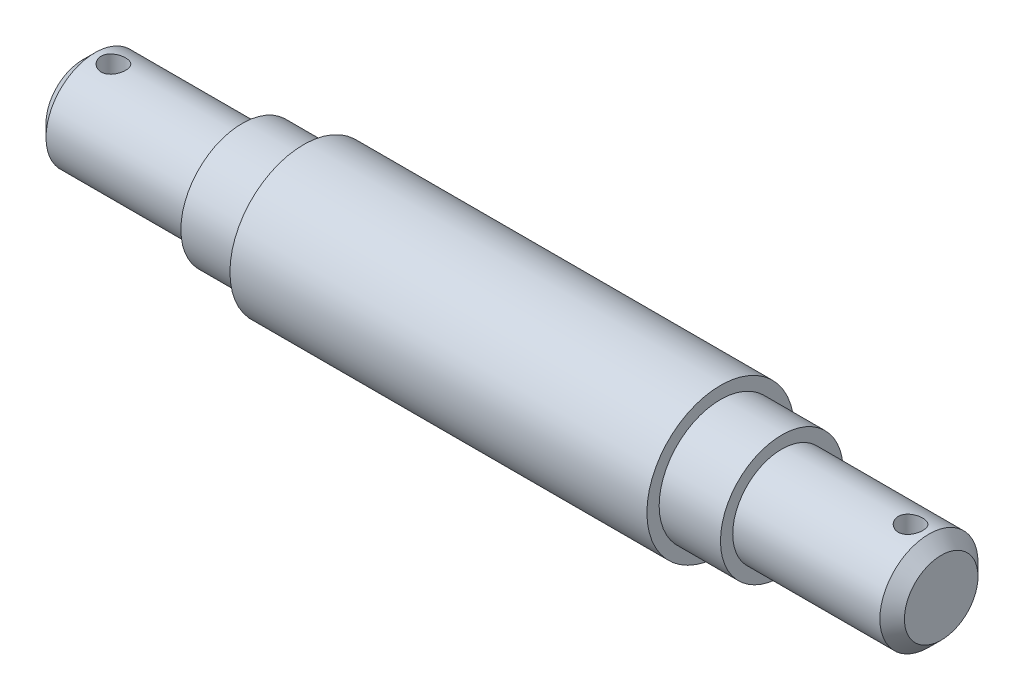
SolidWorks part; units mm, degrees
material "Plain Carbon Steel"
ref_plane "Front Plane" through (0, 0, 0) normal (0, 0, 1) x (1, 0, 0)
ref_plane "Top Plane" through (0, 0, 0) normal (0, 1, 0) x (1, 0, 0)
ref_plane "Right Plane" through (0, 0, 0) normal (1, 0, 0) x (0, 0, -1)
sketch "Shaft Profile Sketch" plane through (0, 0, 0) normal (0, 0, 1) x (1, 0, 0)
  line L0 (0, 0) -> (70, 0)
  line L1 (70, 0) -> (70, -4)
  line L2 (70, -4) -> (57, -4)
  line L3 (57, -4) -> (57, -5)
  line L4 (57, -5) -> (52, -5)
  line L5 (52, -5) -> (52, -6)
  line L6 (52, -6) -> (18, -6)
  line L7 (18, -6) -> (18, -5)
  line L8 (18, -5) -> (13, -5)
  line L9 (13, -5) -> (13, -4)
  line L10 (13, -4) -> (0, -4)
  line L11 (0, -4) -> (0, 0)
  dimension "D1" = 4
  dimension "D2" = 5
  dimension "D3" = 6
  dimension "D4" = 18
  dimension "D5" = 13
  dimension "D6" = 13
  dimension "D7" = 4
  dimension "D8" = 5
  dimension "D9" = 5
  dimension "D10" = 39
revolve "Stepped Shaft Body" add sketch "Shaft Profile Sketch" angle 360 about L0
sketch "Cross Hole Ø2 End 1 Sketch" plane through (0, 0, 0) normal (0, 1, 0) x (1, 0, 0)
  line L0 (13, 4) -> (0, 4) construction
  circle A0 centre (2.5, 0) radius 1
  dimension "D1" = 2
  dimension "D2" = 2.5
  dimension "D3" = 4
extrude "Cross Hole Ø2 End 1" cut sketch "Cross Hole Ø2 End 1 Sketch" against normal mid plane 10
sketch "Cross Hole Ø2 End 2 Sketch" plane through (0, 0, 0) normal (0, 1, 0) x (1, 0, 0)
  line L0 (57, -4) -> (57, 4) construction
  line L2 (57, -4) -> (70, -4) construction
  circle A0 centre (67.5, 0) radius 1
  dimension "D1" = 2
  dimension "D2" = 10.5
  dimension "D3" = 4
extrude "Cross Hole Ø2 End 2" cut sketch "Cross Hole Ø2 End 2 Sketch" against normal mid plane 23
chamfer "End Chamfer 1x45°" distance 1 angle 45 2 edges at (0, 0, 4) (70, 0, 4)
